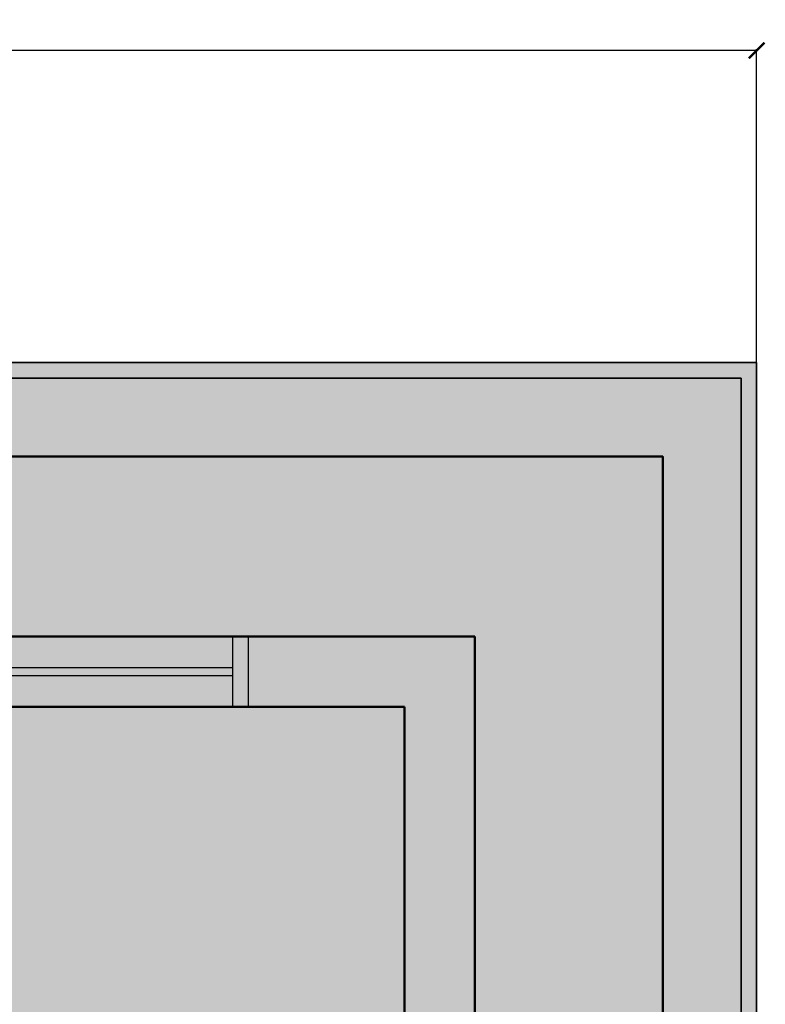
# Model space of a CAD drawing. Units: inches. Extents: x 528 to 2620, y -1066 to 798.
# Tile 19 of 41: x 850 to 945, y 672 to 798. Entities that reach past the tile are written whole.
import ezdxf

# ---------------------------------------------------------------- set-up
doc = ezdxf.new("R2010")
doc.units = ezdxf.units.IN
doc.header["$MEASUREMENT"] = 0
for name, color, linetype, lineweight in [('A-ANNO-DIMS', 2, 'Continuous', 18), ('A-GLAZ', 3, 'Continuous', 25), ('A-WALL', 7, 'Continuous', 50), ('A-WALL-PATT', 8, 'Continuous', 13), ('C-PROP', 5, 'Continuous', 35)]:
    doc.layers.add(name, color=color, linetype=linetype, lineweight=lineweight)
doc.styles.get("Standard").update_dxf_attribs({"font": 'arial.ttf'})
doc.dimstyles.get("Standard").update_dxf_attribs({"dimtxt": 6, "dimasz": 2, "dimexe": 0.18, "dimexo": 0.0625, "dimgap": 0.09, "dimtad": 0, "dimtih": 1, "dimtoh": 1, "dimdec": 1, "dimzin": 0, "dimdsep": 46, "dimlunit": 3, "dimtxsty": 'Standard', "dimblk": 'ARCHTICK', "dimcen": 0.09, "dimadec": 0, "dimazin": 0, "dimtfac": 1, "dimtdec": 1, "dimtofl": 0, "dimtmove": 0, "dimatfit": 3, "dimfxl": 1, "dimtolj": 1, "dimtzin": 0, "dimarcsym": 0})

# ---------------------------------------------------------------- blocks, each defined once
blk = doc.blocks.new('_ArchTick')
at = {"color": 0, "linetype": 'ByBlock', "const_width": 0.15}
blk.add_lwpolyline([(-0.5, -0.5), (0.5, 0.5)], dxfattribs=at)
blk = doc.blocks.new('*D11')
at = {"layer": 'A-ANNO-DIMS', "color": 0, "lineweight": -2, "transparency": 16777216}
for p, q in [((584.06, 753.98), (584.06, 794.01)), ((584.06, 793.83), (758.88, 793.83)), ((944.06, 793.83), (769.24, 793.83)), ((944.06, 753.98), (944.06, 794.01))]:
    blk.add_line(p, q, dxfattribs=at)
at = {"layer": 'Defpoints', "color": 0, "transparency": 16777216}
for p in [(944.06, 793.83), (584.06, 753.92), (944.06, 753.92)]:
    blk.add_point(p, dxfattribs=at)
at = {"layer": 'A-ANNO-DIMS', "color": 0, "lineweight": -2, "transparency": 16777216, "xscale": 2, "yscale": 2, "zscale": 2, "rotation": 180}
blk.add_blockref('_ArchTick', (584.06, 793.83), dxfattribs=at)
at = {"layer": 'A-ANNO-DIMS', "color": 0, "lineweight": -2, "transparency": 16777216, "xscale": 2, "yscale": 2, "zscale": 2}
blk.add_blockref('_ArchTick', (944.06, 793.83), dxfattribs=at)
at = {"layer": 'A-ANNO-DIMS', "color": 0, "transparency": 16777216, "insert": (764.06, 793.83), "char_height": 6, "attachment_point": 5}
blk.add_mtext("\\A1;30'", dxfattribs=at)
blk = doc.blocks.new('WIN-1200')
for p, q in [((677.56, 718.92), (725.56, 718.92)), ((677.56, 709.92), (677.56, 718.92)), ((679.56, 709.92), (679.56, 718.92)), ((723.56, 718.92), (723.56, 709.92)), ((725.56, 718.92), (725.56, 709.92)), ((679.56, 714.92), (723.56, 714.92)), ((679.56, 713.92), (723.56, 713.92)), ((725.56, 709.92), (677.56, 709.92))]:
    blk.add_line(p, q)

msp = doc.modelspace()

# ---------------------------------------------------------------- hatches: boundary and pattern name
at = {"layer": 'A-WALL-PATT', "transparency": 33554687}
h = msp.add_hatch(color=256, dxfattribs=at)
h.dxf.hatch_style = 1
h.paths.add_polyline_path([(944.06, 753.92), (584.06, 753.92), (584.06, 208.92), (608.06, 208.92), (608.06, 210.92), (586.06, 210.92), (586.06, 751.92), (942.06, 751.92), (942.06, 210.92), (728.06, 210.92), (728.06, 208.92), (944.06, 208.92)])
h = msp.add_hatch(color=256, dxfattribs=at)
h.dxf.hatch_style = 1
h.paths.add_polyline_path([(942.06, 751.92), (586.06, 751.92), (586.06, 210.92), (608.06, 210.92), (608.06, 220.92), (596.06, 220.92), (596.06, 741.92), (932.06, 741.92), (932.06, 220.92), (770.06, 220.92), (728.06, 220.92), (728.06, 210.92), (942.06, 210.92)])
at = {"layer": 'A-WALL-PATT', "transparency": 33554475}
h = msp.add_hatch(color=256, dxfattribs=at)
h.dxf.hatch_style = 1
h.paths.add_polyline_path([(620.06, 718.92), (908.06, 718.92), (908.06, 268.92), (770.06, 268.92), (770.06, 220.92), (932.06, 220.92), (932.06, 741.92), (596.06, 741.92), (596.06, 391.42), (620.06, 391.42)])
at = {"layer": 'A-WALL-PATT', "transparency": 33554687}
h = msp.add_hatch(color=256, dxfattribs=at)
h.dxf.hatch_style = 1
h.paths.add_polyline_path([(861.06, 273.92), (817.06, 273.92), (817.06, 272.92), (861.06, 272.92)])
h.paths.add_polyline_path([(817.06, 277.92), (815.06, 277.92), (815.06, 268.92), (817.06, 268.92)])
h.paths.add_polyline_path([(908.06, 397.92), (899.06, 397.92), (899.06, 395.92), (908.06, 395.92)])
h.paths.add_polyline_path([(908.06, 443.92), (899.06, 443.92), (899.06, 441.92), (908.06, 441.92)])
h.paths.add_polyline_path([(904.06, 441.92), (903.06, 441.92), (903.06, 397.92), (904.06, 397.92)])
h.paths.add_polyline_path([(625.06, 561.42), (624.06, 561.42), (624.06, 537.42), (625.06, 537.42)])
h.paths.add_polyline_path([(648.75, 334.44), (720.04, 334.44), (720.04, 345), (648.75, 345)], flags=9)
h.paths.add_polyline_path([(819.73, 323.15), (880.33, 323.15), (880.33, 333.71), (819.73, 333.71)], flags=9)
h.paths.add_polyline_path([(779.9, 680.61), (821.76, 680.61), (821.76, 691.17), (779.9, 691.17)], flags=9)
h.paths.add_polyline_path([(779.88, 692.36), (817.14, 692.36), (817.14, 703.06), (779.88, 703.06)], flags=9)
h.paths.add_polyline_path([(799.99, 453.88), (860.59, 453.88), (860.59, 464.44), (799.99, 464.44)], flags=9)
h.paths.add_polyline_path([(650.87, 539.4), (708.78, 539.4), (708.78, 549.95), (650.87, 549.95)], flags=9)
h.paths.add_polyline_path([(788.5, 612.01), (849.1, 612.01), (849.1, 622.56), (788.5, 622.56)], flags=9)
h.paths.add_polyline_path([(639.54, 648.31), (700.13, 648.31), (700.13, 658.87), (639.54, 658.87)], flags=9)
h.paths.add_polyline_path([(648.91, 346.09), (747.71, 346.09), (747.71, 356.78), (648.91, 356.78)], flags=9)
h.paths.add_polyline_path([(676.86, 450.66), (746.74, 450.66), (746.74, 461.36), (676.86, 461.36)], flags=9)
h.paths.add_polyline_path([(819.71, 334.95), (865.53, 334.95), (865.53, 345.64), (819.71, 345.64)], flags=9)
h.paths.add_polyline_path([(806.3, 467.75), (874.05, 467.75), (874.05, 478.44), (806.3, 478.44)], flags=9)
h.paths.add_polyline_path([(653.23, 552.28), (690.5, 552.28), (690.5, 562.98), (653.23, 562.98)], flags=9)
h.paths.add_polyline_path([(789.9, 623.41), (843.21, 623.41), (843.21, 634.1), (789.9, 634.1)], flags=9)
h.paths.add_polyline_path([(639.77, 662.1), (693.08, 662.1), (693.08, 672.8), (639.77, 672.8)], flags=9)
h.paths.add_polyline_path([(801.59, 242.91), (846.33, 242.91), (846.33, 253.6), (801.59, 253.6)], flags=9)
h.paths.add_polyline_path([(925.36, 593.98), (925.36, 674.06), (914.67, 674.06), (914.67, 593.98)], flags=9)
h.paths.add_polyline_path([(612.56, 593.98), (612.56, 674.06), (601.87, 674.06), (601.87, 593.98)], flags=9)
h.paths.add_polyline_path([(723.31, 726.56), (803.39, 726.56), (803.39, 737.25), (723.31, 737.25)], flags=9)
at = {"layer": 'A-WALL-PATT', "transparency": 33554521}
h = msp.add_hatch(color=256, dxfattribs=at)
h.dxf.hatch_style = 1
h.paths.add_polyline_path([(629.06, 709.92), (677.56, 709.92), (677.56, 718.92), (620.06, 718.92), (620.06, 667.92), (629.06, 667.92)])
h.paths.add_polyline_path([(790.56, 718.92), (725.56, 718.92), (725.56, 709.92), (774.06, 709.92), (774.06, 577.92), (768.48, 577.92), (768.56, 573.42), (774.06, 573.42), (774.06, 567.42), (778.56, 567.42), (778.56, 669.42), (831.06, 669.42), (831.06, 675.92), (826.56, 675.92), (826.56, 673.92), (778.56, 673.92), (778.56, 709.92), (790.56, 709.92)])
h.paths.add_polyline_path([(908.06, 718.92), (879.06, 718.92), (879.06, 709.92), (899.06, 709.92), (899.06, 641.67), (908.06, 641.67)])
h.paths.add_polyline_path([(629.06, 619.92), (620.06, 619.92), (620.06, 561.42), (629.06, 561.42), (629.06, 573.42), (724.06, 573.42), (724.06, 569.42), (728.56, 569.42), (728.56, 577.92), (629.06, 577.92)])
h.paths.add_polyline_path([(779.06, 391.42), (779.06, 400.42), (770.06, 400.42), (764.06, 400.42), (764.06, 397.42), (764.06, 391.42), (770.06, 391.42), (770.06, 268.92), (815.06, 268.92), (815.06, 277.92), (779.06, 277.92), (779.06, 359.77)])
h.paths.add_polyline_path([(908.06, 395.92), (899.06, 395.92), (851.06, 395.92), (851.06, 391.42), (899.06, 391.42), (899.06, 277.92), (863.06, 277.92), (863.06, 268.92), (908.06, 268.92)])
h.paths.add_polyline_path([(908.06, 593.67), (899.06, 593.67), (899.06, 525.42), (778.56, 525.42), (778.56, 527.17), (774.06, 527.17), (774.06, 520.92), (899.06, 520.92), (899.06, 443.92), (908.06, 443.92)])
h.paths.add_polyline_path([(629.06, 520.92), (728.56, 520.92), (728.56, 545.42), (724.06, 545.42), (724.06, 525.42), (629.06, 525.42), (629.06, 537.42), (620.06, 537.42), (620.06, 484.67), (629.06, 484.67)])
h.paths.add_polyline_path([(629.06, 436.67), (620.06, 436.67), (620.06, 391.42), (648.56, 391.42), (648.56, 400.42), (629.06, 400.42)])
h.paths.add_polyline_path([(716.06, 397.42), (716.06, 400.42), (696.56, 400.42), (696.56, 391.42), (716.06, 391.42)])
at = {"layer": 'A-WALL-PATT', "transparency": 33554681}
h = msp.add_hatch(color=256, dxfattribs=at)
h.dxf.hatch_style = 1
h.paths.add_polyline_path([(629.06, 665.92), (625.06, 665.92), (625.06, 621.92), (629.06, 621.92)])
h.paths.add_polyline_path([(624.06, 665.92), (620.06, 665.92), (620.06, 621.92), (624.06, 621.92)])
h.paths.add_polyline_path([(723.56, 713.92), (679.56, 713.92), (679.56, 709.92), (723.56, 709.92)])
h.paths.add_polyline_path([(723.56, 718.92), (679.56, 718.92), (679.56, 714.92), (723.56, 714.92)])
h.paths.add_polyline_path([(814.56, 713.92), (790.56, 713.92), (790.56, 709.92), (814.56, 709.92)])
h.paths.add_polyline_path([(814.56, 718.92), (790.56, 718.92), (790.56, 714.92), (814.56, 714.92)])
h.paths.add_polyline_path([(877.06, 713.92), (833.06, 713.92), (833.06, 709.92), (877.06, 709.92)])
h.paths.add_polyline_path([(877.06, 718.92), (833.06, 718.92), (833.06, 714.92), (877.06, 714.92)])
h.paths.add_polyline_path([(908.06, 639.67), (904.06, 639.67), (904.06, 595.67), (908.06, 595.67)])
h.paths.add_polyline_path([(903.06, 639.67), (899.06, 639.67), (899.06, 595.67), (903.06, 595.67)])
h.paths.add_polyline_path([(908.06, 441.92), (904.06, 441.92), (904.06, 397.92), (908.06, 397.92)])
h.paths.add_polyline_path([(903.06, 441.92), (899.06, 441.92), (899.06, 397.92), (903.06, 397.92)])
h.paths.add_polyline_path([(861.06, 272.92), (817.06, 272.92), (817.06, 268.92), (861.06, 268.92)])
h.paths.add_polyline_path([(861.06, 277.92), (817.06, 277.92), (817.06, 273.92), (861.06, 273.92)])
h.paths.add_polyline_path([(694.56, 395.42), (650.56, 395.42), (650.56, 391.42), (694.56, 391.42)])
h.paths.add_polyline_path([(694.56, 400.42), (650.56, 400.42), (650.56, 396.42), (694.56, 396.42)])
h.paths.add_polyline_path([(629.06, 482.67), (625.06, 482.67), (625.06, 438.67), (629.06, 438.67)])
h.paths.add_polyline_path([(624.06, 482.67), (620.06, 482.67), (620.06, 438.67), (624.06, 438.67)])
h.paths.add_polyline_path([(629.06, 561.42), (625.06, 561.42), (625.06, 537.42), (629.06, 537.42)])
h.paths.add_polyline_path([(624.06, 561.42), (620.06, 561.42), (620.06, 537.42), (624.06, 537.42)])
h = msp.add_hatch(color=256, dxfattribs=at)
h.dxf.hatch_style = 1
h.paths.add_polyline_path([(625.06, 665.92), (624.06, 665.92), (624.06, 621.92), (625.06, 621.92)])
h.paths.add_polyline_path([(629.06, 667.92), (620.06, 667.92), (620.06, 665.92), (629.06, 665.92)])
h.paths.add_polyline_path([(629.06, 621.92), (620.06, 621.92), (620.06, 619.92), (629.06, 619.92)])
h.paths.add_polyline_path([(723.56, 714.92), (679.56, 714.92), (679.56, 713.92), (723.56, 713.92)])
h.paths.add_polyline_path([(725.56, 718.92), (723.56, 718.92), (723.56, 709.92), (725.56, 709.92)])
h.paths.add_polyline_path([(679.56, 718.92), (677.56, 718.92), (677.56, 709.92), (679.56, 709.92)])
h.paths.add_polyline_path([(814.56, 714.92), (790.56, 714.92), (790.56, 713.92), (814.56, 713.92)])
h.paths.add_polyline_path([(877.06, 714.92), (833.06, 714.92), (833.06, 713.92), (877.06, 713.92)])
h.paths.add_polyline_path([(879.06, 718.92), (877.06, 718.92), (877.06, 709.92), (879.06, 709.92)])
h.paths.add_polyline_path([(833.06, 718.92), (831.06, 718.92), (831.06, 709.92), (833.06, 709.92)])
h.paths.add_polyline_path([(650.56, 400.42), (648.56, 400.42), (648.56, 391.42), (650.56, 391.42)])
h.paths.add_polyline_path([(694.56, 396.42), (650.56, 396.42), (650.56, 395.42), (694.56, 395.42)])
h.paths.add_polyline_path([(696.56, 400.42), (694.56, 400.42), (694.56, 391.42), (696.56, 391.42)])
h.paths.add_polyline_path([(629.06, 438.67), (620.06, 438.67), (620.06, 436.67), (629.06, 436.67)])
h.paths.add_polyline_path([(629.06, 484.67), (620.06, 484.67), (620.06, 482.67), (629.06, 482.67)])
h.paths.add_polyline_path([(625.06, 482.67), (624.06, 482.67), (624.06, 438.67), (625.06, 438.67)])
at = {"layer": 'A-WALL-PATT', "transparency": 33554590}
h = msp.add_hatch(color=256, dxfattribs=at)
h.dxf.hatch_style = 1
h.paths.add_polyline_path([(774.06, 709.92), (629.06, 709.92), (629.06, 577.92), (728.56, 577.92), (728.56, 579.42), (728.56, 619.42), (730.31, 619.42), (730.31, 619.38, -0.401453), (768.56, 579.42), (768.56, 577.92), (774.06, 577.92)])
h.paths.add_polyline_path([(723.9, 686.06), (723.97, 686.06), (723.83, 686.13)], flags=0)
h.paths.add_polyline_path([(722.79, 642.7), (722.89, 642.76), (722.89, 684.99), (722.65, 685.24), (722.65, 685.82), (723.08, 686.26), (723.53, 686.26), (723.97, 686.06), (724.74, 686.13), (770.7, 686.13), (770.78, 686.14), (771.13, 686.27), (771.69, 686.09), (771.94, 685.48), (771.67, 684.9), (771.58, 684.87), (771.58, 642.78), (771.88, 642.51), (771.88, 641.92), (771.51, 641.46), (770.85, 641.46), (770.4, 641.83), (770.4, 641.55), (724.74, 641.55), (723.99, 641.7), (723.44, 641.41), (722.88, 641.59), (722.6, 642.14)], flags=16)
h.paths.add_polyline_path([(723.99, 641.7), (723.99, 641.71), (723.99, 641.7)], flags=0)
h.paths.add_polyline_path([(722.89, 642.73), (722.89, 684.99), (722.65, 685.24), (722.65, 685.82), (723.08, 686.26), (723.29, 686.26), (722.99, 686.17), (722.79, 685.97), (722.65, 685.68), (722.65, 685.43), (722.75, 685.14), (722.94, 684.94), (723.24, 684.81), (723.48, 684.81), (723.78, 684.9), (723.98, 685.1), (724.17, 685.49), (724.12, 685.64), (724.12, 685.25), (723.63, 684.75), (723.63, 642.96), (724.12, 642.51), (724.12, 641.89), (723.66, 641.46), (723.08, 641.46), (722.65, 641.9), (722.65, 642.48)], flags=0)
h.paths.add_polyline_path([(722.65, 642.29), (722.65, 642.04), (722.79, 641.75), (723.08, 641.46), (723.29, 641.46), (722.88, 641.59), (722.6, 642.14)], flags=0)
h.paths.add_polyline_path([(770.75, 686.13), (770.58, 686.13), (770.55, 686.06)], flags=0)
h.paths.add_polyline_path([(743.3, 645.29), (753.23, 659.4), (748.69, 663.75), (753.23, 668.54), (743.3, 682.46), (743.79, 682.59), (744.14, 682.68), (744.53, 682.93), (744.63, 683.08), (745.02, 683.33), (744.53, 684.07), (744.78, 684.16), (744.87, 684.31), (745.51, 684.4), (746.08, 684.65), (746.47, 684.65), (746.82, 684.81), (747.46, 685.03), (747.71, 685.14), (748.2, 685.28), (748.39, 685.52), (748.86, 685.52), (749.99, 686.13), (753.49, 676.03), (757.38, 680.15), (757.79, 679.76), (758.04, 680.65), (758.29, 681.23), (758.29, 682.05), (758.02, 682.59), (757.87, 683.17), (757.82, 683.78), (758.39, 684.07), (758.98, 684.2), (759.62, 684.16), (760.21, 683.96), (760.75, 683.67), (761.86, 683.67), (762.4, 683.96), (762.99, 684.11), (763.63, 684.11), (764.2, 683.96), (764.74, 683.67), (766.12, 683.67), (766.66, 683.96), (767.25, 684.16), (767.87, 684.2), (768.46, 684.07), (769.05, 683.78), (769, 683.17), (768.85, 682.59), (768.55, 682.05), (768.55, 681.23), (768.8, 680.65), (769.09, 679.75), (768.95, 678.83), (768.8, 678.23), (768.55, 677.65), (768.55, 676.82), (768.8, 676.24), (769.09, 675.34), (768.95, 674.42), (768.8, 673.82), (768.55, 673.28), (768.55, 672.41), (768.8, 671.87), (769, 671.29), (769.05, 670.64), (768.95, 670.02), (768.8, 669.41), (768.55, 668.87), (768.55, 668), (768.97, 667.24), (769.05, 666.28), (769.05, 665.56), (768.46, 665.32), (767.87, 665.16), (767.25, 665.16), (766.66, 665.36), (766.12, 665.7), (764.74, 665.7), (763.94, 665.2), (762.99, 665.2), (762.4, 665.36), (761.86, 665.7), (761, 665.7), (762.7, 664.09), (760.74, 662.03), (761.86, 662.03), (762.4, 662.32), (763.34, 662.55), (764.25, 662.32), (764.79, 662.03), (766.12, 662.03), (766.66, 662.32), (767.25, 662.52), (767.87, 662.56), (768.51, 662.43), (769.05, 662.12), (769.05, 661.4), (769.05, 660.8), (768.85, 660.21), (768.55, 659.68), (768.55, 658.85), (768.85, 658.27), (769, 657.66), (769.07, 656.75), (768.85, 655.85), (768.55, 655.27), (768.55, 654.44), (768.85, 653.86), (769.07, 652.96), (769, 652.05), (768.85, 651.44), (768.55, 650.91), (768.55, 650.03), (768.85, 649.5), (769, 648.91), (769.05, 648.26), (769, 647.64), (768.85, 647.03), (768.55, 646.5), (768.55, 645.62), (768.85, 645.09), (769.05, 644.55), (769.05, 643.9), (768.51, 643.65), (767.87, 643.52), (767.25, 643.52), (766.66, 643.72), (766.12, 644.06), (764.79, 644.06), (764.25, 643.72), (763.34, 643.49), (762.4, 643.72), (761.86, 644.06), (760.8, 644.06), (760.26, 643.72), (759.67, 643.52), (759.03, 643.52), (758.39, 643.65), (757.87, 643.9), (757.87, 644.55), (758.04, 645.09), (758.34, 645.62), (758.34, 646.5), (758.04, 647.03), (757.92, 647.64), (757.87, 648.06), (757.38, 647.59), (753.42, 651.77), (749.99, 641.62), (749.5, 641.71), (749.35, 641.95), (748.54, 642.45), (747.31, 642.94), (746.65, 642.94), (746.33, 643.18), (745.51, 643.57), (744.53, 643.65), (745.01, 644.4), (744.63, 644.64), (744.14, 644.89), (743.79, 645.13)], flags=0)
h.paths.add_polyline_path([(755.66, 654.93), (756.54, 654.69), (757.53, 654.33), (756.64, 654.58)], flags=0)
h.paths.add_polyline_path([(758.34, 649.2), (758.34, 648.71), (758.59, 644.3), (758.59, 648.8)], flags=0)
h.paths.add_polyline_path([(758.34, 649.29), (758.09, 649.7), (758.36, 649.17)], flags=0)
h.paths.add_polyline_path([(755.66, 672.79), (756.49, 673.04), (757.36, 673.35), (757.35, 673.36), (756.64, 673.15)], flags=0)
h.paths.add_polyline_path([(760.26, 639.64), (771.41, 639.64), (771.41, 624.04), (760.26, 624.04)], flags=16)
h.paths.add_polyline_path([(761.38, 638.53), (770.29, 638.53), (770.29, 625.15), (761.38, 625.15)], flags=0)
edge = h.paths.add_edge_path(flags=0)
edge.add_ellipse((765.84, 631.84), major_axis=(-2.24, 2.24), ratio=1, start_angle=-45, end_angle=45, ccw=False)
edge.add_ellipse((765.84, 631.84), major_axis=(-2.24, 2.24), ratio=1, start_angle=-135, end_angle=-45, ccw=False)
edge.add_ellipse((765.84, 631.84), major_axis=(-2.24, 2.24), ratio=1, start_angle=135, end_angle=-135, ccw=False)
edge.add_ellipse((765.84, 631.84), major_axis=(-2.24, 2.24), ratio=1, start_angle=45, end_angle=135, ccw=False)
h.paths.add_polyline_path([(758.59, 683.42), (758.59, 678.92), (758.37, 678.58), (758.34, 678.43), (758.09, 678.05), (758.34, 678.52), (758.34, 679.01)], flags=0)
h.paths.add_polyline_path([(760.26, 688.04), (760.26, 703.64), (771.41, 703.64), (771.41, 688.04)], flags=16)
h.paths.add_polyline_path([(770.4, 685.39), (770.4, 685.85), (770.85, 686.22), (771.51, 686.22), (771.88, 685.76), (771.88, 685.17), (771.58, 684.9), (771.58, 642.78), (771.88, 642.51), (771.88, 641.92), (771.51, 641.46), (770.85, 641.46), (770.4, 641.83), (770.4, 642.29)], flags=0)
h.paths.add_polyline_path([(770.53, 642.68), (771.05, 643.01), (771.67, 642.77), (771.94, 642.2), (771.69, 641.59), (771.13, 641.41), (770.55, 641.62), (770.35, 642.13)], flags=16)
h.paths.add_polyline_path([(761.38, 689.15), (761.38, 702.53), (770.29, 702.53), (770.29, 689.15)], flags=0)
edge = h.paths.add_edge_path(flags=0)
edge.add_ellipse((765.84, 695.84), major_axis=(2.24, 2.24), ratio=1, start_angle=405, end_angle=495, ccw=False)
edge.add_ellipse((765.84, 695.84), major_axis=(2.24, 2.24), ratio=1, start_angle=675, end_angle=765, ccw=False)
edge.add_ellipse((765.84, 695.84), major_axis=(2.24, 2.24), ratio=1, start_angle=585, end_angle=675, ccw=False)
edge.add_ellipse((765.84, 695.84), major_axis=(2.24, 2.24), ratio=1, start_angle=495, end_angle=585, ccw=False)
h.paths.add_polyline_path([(770.7, 684.9), (770.94, 684.74), (771.41, 684.74), (771.73, 685.03), (771.88, 685.34), (771.88, 685.64), (771.69, 686.09), (771.58, 686.13), (771.88, 685.76), (771.88, 685.17), (771.41, 684.74), (770.85, 684.74)], flags=0)
h.paths.add_polyline_path([(899.06, 709.92), (831.06, 709.92), (831.06, 699.92), (829.81, 699.92), (829.81, 675.92), (831.06, 675.92), (831.06, 669.42), (778.56, 669.42), (778.56, 567.17), (780.06, 567.17), (820.06, 567.17), (820.06, 565.42), (820.02, 565.42, -0.401453), (780.06, 527.17), (778.56, 527.17), (778.56, 525.42), (899.06, 525.42)])
h.paths.add_polyline_path([(849.2, 636.01), (849.27, 636.02), (849.13, 636.08)], flags=0)
h.paths.add_polyline_path([(848.19, 634.95), (847.95, 635.2), (847.95, 635.78), (848.38, 636.22), (848.83, 636.22), (849.27, 636.02), (850.04, 636.08), (896, 636.08), (896.08, 636.1), (896.43, 636.22), (896.99, 636.05), (897.24, 635.43), (896.97, 634.86), (896.88, 634.83), (896.88, 592.74), (897.18, 592.47), (897.18, 591.88), (896.81, 591.42), (896.15, 591.42), (895.7, 591.79), (895.7, 591.51), (850.04, 591.51), (849.29, 591.66), (848.74, 591.37), (848.18, 591.54), (847.9, 592.1), (848.09, 592.65), (848.19, 592.71)], flags=16)
h.paths.add_polyline_path([(849.29, 591.66), (849.29, 591.66), (849.29, 591.66)], flags=16)
h.paths.add_polyline_path([(848.19, 634.95), (847.95, 635.2), (847.95, 635.78), (848.38, 636.22), (848.59, 636.22), (848.29, 636.13), (848.09, 635.93), (847.95, 635.64), (847.95, 635.39), (848.05, 635.1), (848.24, 634.9), (848.54, 634.76), (848.78, 634.76), (849.08, 634.85), (849.28, 635.05), (849.47, 635.44), (849.42, 635.59), (849.42, 635.21), (848.93, 634.7), (848.93, 592.92), (849.42, 592.47), (849.42, 591.84), (848.96, 591.42), (848.38, 591.42), (847.95, 591.86), (847.95, 592.44), (848.19, 592.69)], flags=0)
h.paths.add_polyline_path([(847.95, 592.25), (847.95, 592), (848.09, 591.71), (848.38, 591.42), (848.59, 591.42), (848.18, 591.54), (847.9, 592.1)], flags=16)
h.paths.add_polyline_path([(896.05, 636.08), (895.88, 636.08), (895.85, 636.01)], flags=0)
h.paths.add_polyline_path([(868.6, 632.41), (869.09, 632.55), (869.44, 632.64), (869.83, 632.88), (869.93, 633.04), (870.32, 633.28), (869.83, 634.02), (870.08, 634.11), (870.17, 634.27), (870.81, 634.36), (871.38, 634.61), (871.77, 634.61), (872.12, 634.76), (872.76, 634.99), (873.01, 635.1), (873.5, 635.23), (873.69, 635.48), (874.16, 635.48), (875.29, 636.08), (878.79, 625.99), (882.68, 630.11), (883.09, 629.71), (883.34, 630.6), (883.59, 631.18), (883.59, 632.01), (883.32, 632.55), (883.17, 633.13), (883.12, 633.73), (883.69, 634.02), (884.28, 634.16), (884.92, 634.11), (885.51, 633.91), (886.05, 633.62), (887.16, 633.62), (887.7, 633.91), (888.29, 634.07), (888.93, 634.07), (889.5, 633.91), (890.04, 633.62), (891.42, 633.62), (891.96, 633.91), (892.55, 634.11), (893.17, 634.16), (893.76, 634.02), (894.35, 633.73), (894.3, 633.13), (894.15, 632.55), (893.85, 632.01), (893.85, 631.18), (894.1, 630.6), (894.39, 629.71), (894.25, 628.79), (894.1, 628.18), (893.85, 627.6), (893.85, 626.77), (894.1, 626.19), (894.39, 625.3), (894.25, 624.38), (894.1, 623.78), (893.85, 623.24), (893.85, 622.37), (894.1, 621.83), (894.3, 621.25), (894.35, 620.6), (894.25, 619.97), (894.1, 619.37), (893.85, 618.83), (893.85, 617.96), (894.27, 617.2), (894.35, 616.23), (894.35, 615.52), (893.76, 615.27), (893.17, 615.12), (892.55, 615.12), (891.96, 615.32), (891.42, 615.65), (890.04, 615.65), (889.25, 615.16), (888.29, 615.16), (887.7, 615.32), (887.16, 615.65), (886.31, 615.65), (888, 614.04), (886.04, 611.98), (887.16, 611.98), (887.7, 612.27), (888.64, 612.5), (889.55, 612.27), (890.09, 611.98), (891.42, 611.98), (891.96, 612.27), (892.55, 612.48), (893.17, 612.52), (893.81, 612.39), (894.35, 612.07), (894.35, 611.36), (894.35, 610.75), (894.15, 610.17), (893.85, 609.63), (893.85, 608.81), (894.15, 608.22), (894.3, 607.62), (894.37, 606.7), (894.15, 605.81), (893.85, 605.22), (893.85, 604.4), (894.15, 603.81), (894.37, 602.92), (894.3, 602), (894.15, 601.4), (893.85, 600.86), (893.85, 599.99), (894.15, 599.45), (894.3, 598.87), (894.35, 598.22), (894.3, 597.59), (894.15, 596.99), (893.85, 596.45), (893.85, 595.58), (894.15, 595.04), (894.35, 594.51), (894.35, 593.86), (893.81, 593.61), (893.17, 593.48), (892.55, 593.48), (891.96, 593.68), (891.42, 594.01), (890.09, 594.01), (889.55, 593.68), (888.64, 593.45), (887.7, 593.68), (887.16, 594.01), (886.1, 594.01), (885.56, 593.68), (884.97, 593.48), (884.33, 593.48), (883.69, 593.61), (883.17, 593.86), (883.17, 594.51), (883.34, 595.04), (883.64, 595.58), (883.64, 596.45), (883.34, 596.99), (883.22, 597.59), (883.17, 598.01), (882.68, 597.55), (878.72, 601.73), (875.29, 591.57), (874.8, 591.66), (874.65, 591.91), (873.84, 592.4), (872.61, 592.89), (871.95, 592.89), (871.63, 593.14), (870.81, 593.52), (869.83, 593.61), (870.31, 594.36), (869.93, 594.6), (869.44, 594.84), (869.09, 595.09), (868.6, 595.24), (878.53, 609.35), (873.99, 613.71), (878.53, 618.49)], flags=0)
h.paths.add_polyline_path([(880.96, 622.75), (881.79, 622.99), (882.66, 623.31), (882.65, 623.31), (881.94, 623.1)], flags=0)
h.paths.add_polyline_path([(880.96, 604.89), (881.84, 604.64), (882.83, 604.28), (881.94, 604.53)], flags=16)
h.paths.add_polyline_path([(883.39, 628.01), (883.64, 628.48), (883.64, 628.97), (883.89, 633.38), (883.89, 628.88), (883.67, 628.53), (883.64, 628.39)], flags=0)
h.paths.add_polyline_path([(883.64, 599.16), (883.64, 598.67), (883.89, 594.26), (883.89, 598.76)], flags=16)
h.paths.add_polyline_path([(883.64, 599.25), (883.39, 599.65), (883.66, 599.12)], flags=16)
h.paths.add_polyline_path([(885.56, 637.99), (885.56, 653.6), (896.71, 653.6), (896.71, 637.99)], flags=16)
h.paths.add_polyline_path([(885.56, 589.6), (896.71, 589.6), (896.71, 573.99), (885.56, 573.99)], flags=16)
h.paths.add_polyline_path([(886.68, 639.11), (886.68, 652.48), (895.59, 652.48), (895.59, 639.11)], flags=0)
h.paths.add_polyline_path([(886.68, 588.48), (895.59, 588.48), (895.59, 575.11), (886.68, 575.11)], flags=0)
edge = h.paths.add_edge_path(flags=0)
edge.add_ellipse((891.14, 645.79), major_axis=(2.24, 2.24), ratio=1, start_angle=405, end_angle=495, ccw=False)
edge.add_ellipse((891.14, 645.79), major_axis=(2.24, 2.24), ratio=1, start_angle=675, end_angle=765, ccw=False)
edge.add_ellipse((891.14, 645.79), major_axis=(2.24, 2.24), ratio=1, start_angle=585, end_angle=675, ccw=False)
edge.add_ellipse((891.14, 645.79), major_axis=(2.24, 2.24), ratio=1, start_angle=495, end_angle=585, ccw=False)
edge = h.paths.add_edge_path(flags=0)
edge.add_ellipse((891.14, 581.8), major_axis=(-2.24, 2.24), ratio=1, start_angle=-45, end_angle=45, ccw=False)
edge.add_ellipse((891.14, 581.8), major_axis=(-2.24, 2.24), ratio=1, start_angle=-135, end_angle=-45, ccw=False)
edge.add_ellipse((891.14, 581.8), major_axis=(-2.24, 2.24), ratio=1, start_angle=135, end_angle=-135, ccw=False)
edge.add_ellipse((891.14, 581.8), major_axis=(-2.24, 2.24), ratio=1, start_angle=45, end_angle=135, ccw=False)
h.paths.add_polyline_path([(895.7, 635.35), (895.7, 635.8), (896.15, 636.17), (896.81, 636.17), (897.18, 635.71), (897.18, 635.12), (896.88, 634.85), (896.88, 592.74), (897.18, 592.47), (897.18, 591.88), (896.81, 591.42), (896.15, 591.42), (895.7, 591.79), (895.7, 592.25)], flags=0)
h.paths.add_polyline_path([(896, 634.85), (896.24, 634.7), (896.71, 634.7), (897.03, 634.99), (897.18, 635.3), (897.18, 635.59), (896.99, 636.05), (896.88, 636.08), (897.18, 635.71), (897.18, 635.12), (896.71, 634.7), (896.15, 634.7)], flags=0)
h.paths.add_polyline_path([(895.83, 592.63), (896.35, 592.96), (896.97, 592.73), (897.24, 592.16), (896.99, 591.54), (896.43, 591.37), (895.85, 591.58), (895.65, 592.09)], flags=16)
h.paths.add_polyline_path([(725.25, 569.42), (724.06, 569.42), (724.06, 573.42), (629.06, 573.42), (629.06, 525.42), (724.06, 525.42), (724.06, 545.42), (725.25, 545.42)])
h.paths.add_polyline_path([(820.02, 565.42), (780.06, 565.42), (780.06, 567.17), (774.06, 567.17), (774.06, 567.42), (774.06, 573.42), (768.56, 573.42), (768.48, 577.92), (768.56, 577.92), (768.56, 579.42, 0.401453), (730.31, 619.38), (730.31, 579.42), (728.56, 579.42), (728.56, 573.42), (728.56, 569.42), (727.25, 569.42), (727.25, 545.42), (728.56, 545.42), (728.56, 520.92), (665.06, 520.92), (665.06, 436.42), (716.06, 436.42), (716.06, 421.42), (717.81, 421.42), (717.81, 421.36, -0.392996), (740.06, 397.42, -0.392996), (762.31, 421.36), (762.31, 421.42), (764.06, 421.42), (764.06, 400.42), (770.06, 400.42), (779.06, 400.42), (779.06, 391.42), (779.06, 359.77), (795.43, 359.77), (795.43, 294.3), (893.67, 294.3), (893.67, 277.92), (899.06, 277.92), (899.06, 391.42), (851.06, 391.42), (851.06, 395.92), (899.06, 395.92), (899.06, 443.92), (899.06, 520.92), (774.06, 520.92), (774.06, 527.17), (778.56, 527.17), (780.06, 527.17, 0.401453)])
h.paths.add_polyline_path([(774.06, 519.66), (842.12, 519.66), (842.12, 505.07), (788.64, 505.07), (788.64, 474.08), (788.64, 470.43, -0.883215), (779.53, 456.66), (774.97, 456.66, -0.414214), (774.06, 457.57)], flags=16)
h.paths.add_polyline_path([(775.88, 517.83), (840.3, 517.83), (840.3, 514.19), (788.64, 514.19), (788.64, 484.41), (779.53, 484.41), (779.53, 474.08), (775.88, 474.08)], flags=0)
h.paths.add_polyline_path([(706.7, 501.56, -0.254069), (706.7, 493.02), (698.31, 492.55), (698.31, 502.03)], flags=16)
h.paths.add_polyline_path([(691.33, 515.69), (691.8, 507.3), (682.32, 507.3), (682.79, 515.69, -0.254069)], flags=16)
h.paths.add_polyline_path([(695.49, 504.68), (695.49, 479.42), (678.64, 479.42), (678.64, 504.68)], flags=16)
h.paths.add_polyline_path([(706.7, 489.6, -0.254069), (706.7, 481.06), (698.31, 480.59), (698.31, 490.07)], flags=16)
h.paths.add_polyline_path([(675.81, 502.03), (675.81, 492.55), (667.42, 493.02, -0.254069), (667.42, 501.56)], flags=16)
h.paths.add_polyline_path([(691.8, 476.8), (691.33, 468.41, -0.254069), (682.79, 468.41), (682.32, 476.8)], flags=16)
h.paths.add_polyline_path([(675.81, 490.07), (675.81, 480.59), (667.42, 481.06, -0.254069), (667.42, 489.6)], flags=16)
h.paths.add_polyline_path([(764.06, 397.42), (762.31, 397.42), (762.31, 421.36, 0.392996), (740.06, 397.42, 0.392996), (717.81, 421.36), (717.81, 397.42), (716.06, 397.42), (716.06, 391.42), (716.06, 385.42), (764.06, 385.42), (764.06, 391.42)], flags=17)
h.paths.add_polyline_path([(716.06, 436.42), (705.86, 436.42), (705.86, 418.42), (716.06, 418.42), (716.06, 421.42)], flags=17)
h.paths.add_polyline_path([(716.06, 418.42), (705.86, 418.42), (705.86, 400.42), (716.06, 400.42)], flags=17)
h.paths.add_polyline_path([(705.86, 418.42), (695.66, 418.42), (695.66, 400.42), (696.56, 400.42), (705.86, 400.42)], flags=17)
h.paths.add_polyline_path([(705.86, 436.42), (695.66, 436.42), (695.66, 418.42), (705.86, 418.42)], flags=17)
h.paths.add_polyline_path([(695.66, 418.42), (685.46, 418.42), (685.46, 400.42), (695.66, 400.42)], flags=17)
h.paths.add_polyline_path([(695.66, 436.42), (685.46, 436.42), (685.46, 418.42), (695.66, 418.42)], flags=17)
h.paths.add_polyline_path([(685.46, 418.42), (675.26, 418.42), (675.26, 400.42), (685.46, 400.42)], flags=17)
h.paths.add_polyline_path([(685.46, 436.42), (675.26, 436.42), (675.26, 418.42), (685.46, 418.42)], flags=17)
h.paths.add_polyline_path([(675.26, 436.42), (665.06, 436.42), (665.06, 418.42), (675.26, 418.42)])
h.paths.add_polyline_path([(675.26, 418.42), (665.06, 418.42), (665.06, 400.42), (675.26, 400.42)])
h.paths.add_polyline_path([(665.06, 418.42), (646.97, 418.42), (646.99, 436.42), (629.06, 436.42), (629.06, 400.42), (665.06, 400.42)])
h.paths.add_polyline_path([(665.06, 436.42), (646.99, 436.42), (646.97, 418.42), (665.06, 418.42)], flags=17)
h.paths.add_polyline_path([(647.01, 446.62), (629.06, 446.62), (629.06, 436.67), (629.06, 436.42), (646.99, 436.42)])
h.paths.add_polyline_path([(665.06, 446.62), (647.01, 446.62), (646.99, 436.42), (665.06, 436.42)])
h.paths.add_polyline_path([(647.02, 456.82), (629.06, 456.82), (629.06, 446.62), (647.01, 446.62)])
h.paths.add_polyline_path([(665.06, 456.82), (647.02, 456.82), (647.01, 446.62), (665.06, 446.62)])
h.paths.add_polyline_path([(647.03, 467.02), (629.06, 467.02), (629.06, 456.82), (647.02, 456.82)])
h.paths.add_polyline_path([(665.06, 467.02), (647.03, 467.02), (647.02, 456.82), (665.06, 456.82)])
h.paths.add_polyline_path([(665.06, 477.22), (647.05, 477.22), (647.03, 467.02), (665.06, 467.02)])
h.paths.add_polyline_path([(647.05, 477.22), (629.06, 477.22), (629.06, 467.02), (647.03, 467.02)])
h.paths.add_polyline_path([(647.06, 487.22), (629.06, 487.22), (629.06, 477.22), (647.05, 477.22), (647.05, 479.02), (645.53, 483.25), (640.88, 480.37)])
h.paths.add_polyline_path([(665.06, 520.92), (629.06, 520.92), (629.06, 487.22), (647.06, 487.22), (665.06, 487.22)])
h.paths.add_polyline_path([(665.06, 487.22), (647.06, 487.22), (653.22, 480.35), (648.58, 483.24), (647.05, 479.02), (647.05, 477.22), (665.06, 477.22)])

# ---------------------------------------------------------------- linework, layer by layer
at = {"layer": 'A-WALL'}
for p, q in [((932.06, 741.92), (596.06, 741.92)), ((932.06, 220.92), (932.06, 741.92)), ((908.06, 718.92), (620.06, 718.92)), ((908.06, 268.92), (908.06, 718.92)), ((899.06, 709.92), (831.06, 709.92)), ((899.06, 709.92), (831.06, 709.92)), ((899.06, 525.42), (899.06, 709.92))]:
    msp.add_line(p, q, dxfattribs=at)
at = {"layer": 'C-PROP'}
for points in [[(728.06, 208.92), (944.06, 208.92), (944.06, 753.92), (584.06, 753.92), (584.06, 208.92), (608.06, 208.92)], [(728.06, 210.92), (942.06, 210.92), (942.06, 751.92), (586.06, 751.92), (586.06, 210.92), (608.06, 210.92)]]:
    msp.add_lwpolyline(points, dxfattribs=at)
msp.add_lwpolyline([(596.06, 741.92), (596.06, 220.92), (932.06, 220.92), (932.06, 741.92)], close=True, dxfattribs=at)

# ---------------------------------------------------------------- block references
at = {"layer": 'A-GLAZ'}
msp.add_blockref('WIN-1200', (153.5, 0), dxfattribs=at)

# ---------------------------------------------------------------- dimensions: what is measured, and where the dimension line sits
at = {"layer": 'A-ANNO-DIMS'}
dim = msp.add_linear_dim(base=(944.06, 793.83), p1=(584.06, 753.92), p2=(944.06, 753.92), dimstyle='Standard', override={"dimclrd": 0, "dimclre": 0, "dimclrt": 0}, dxfattribs=at)
dim.commit()
dim.dimension.update_dxf_attribs({"geometry": '*D11', "text_midpoint": (764.06, 793.83)})

doc.saveas('drawing.dxf')
